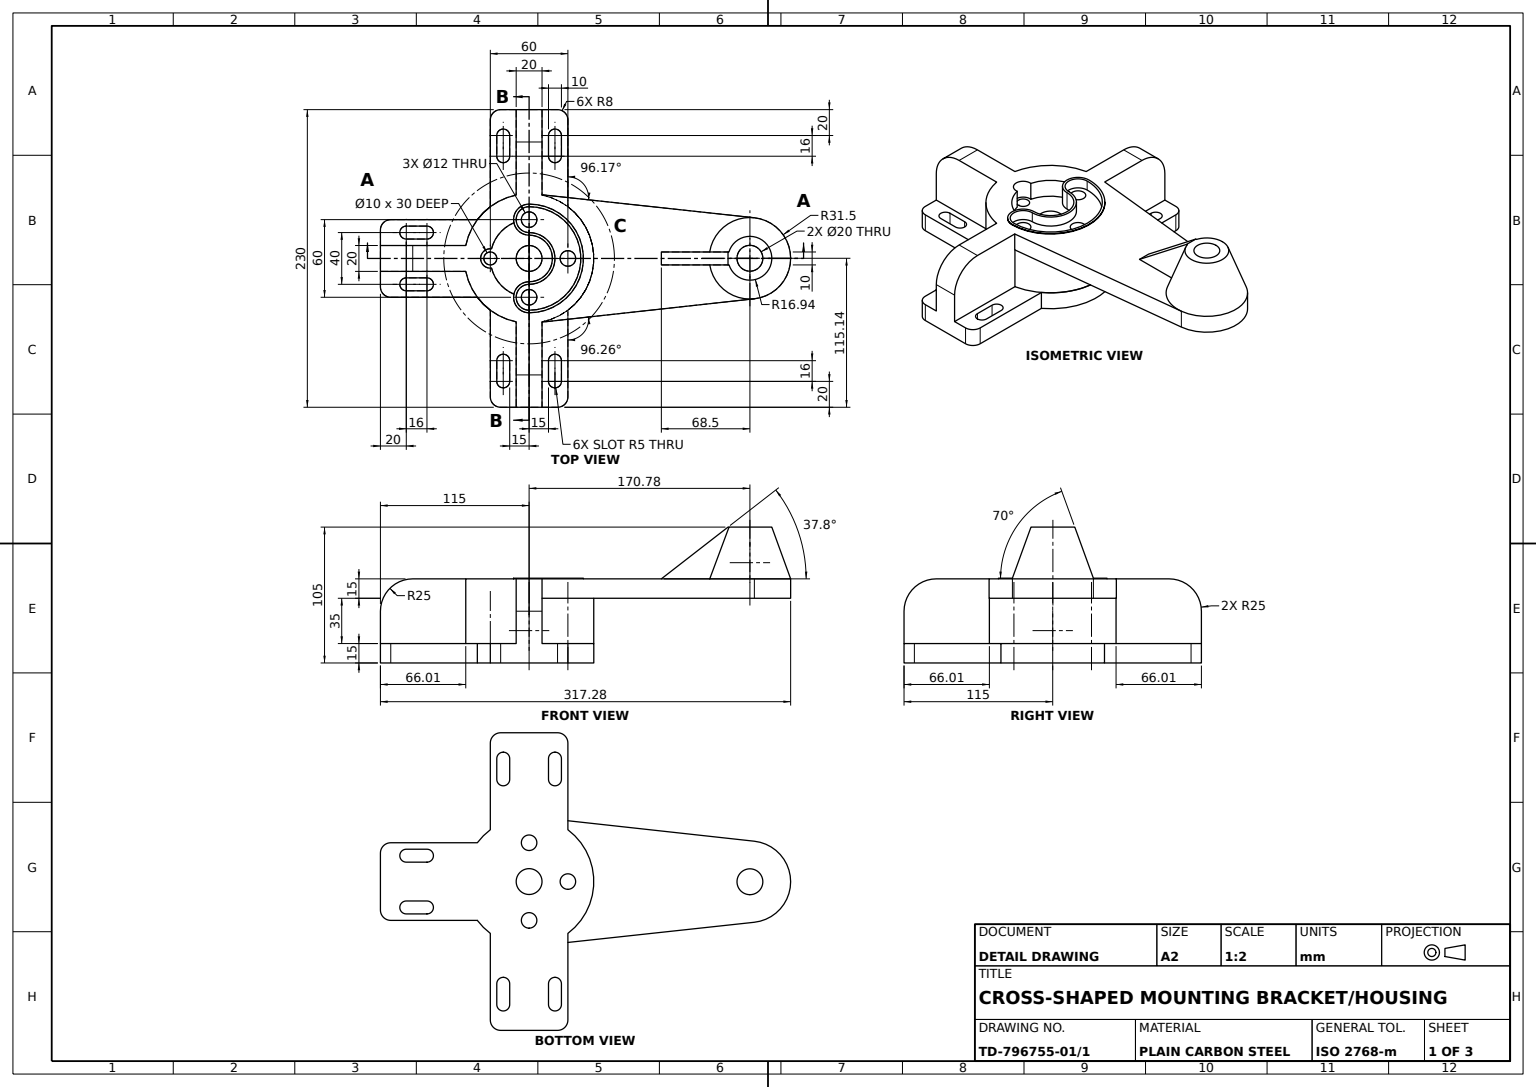
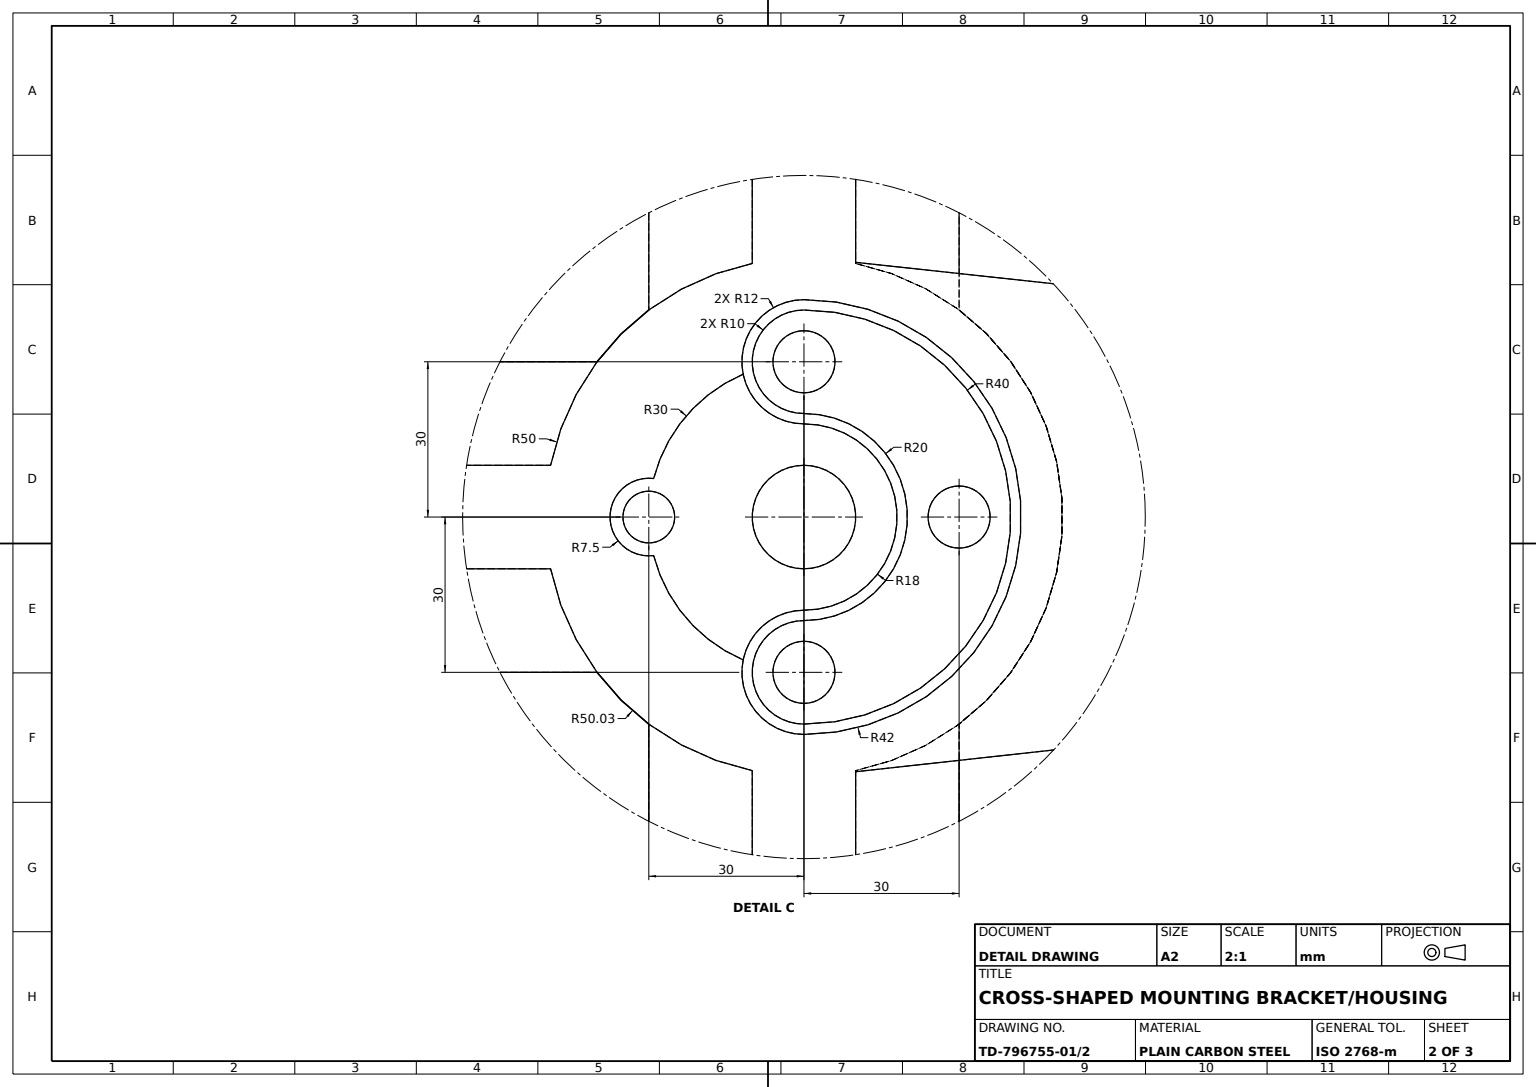
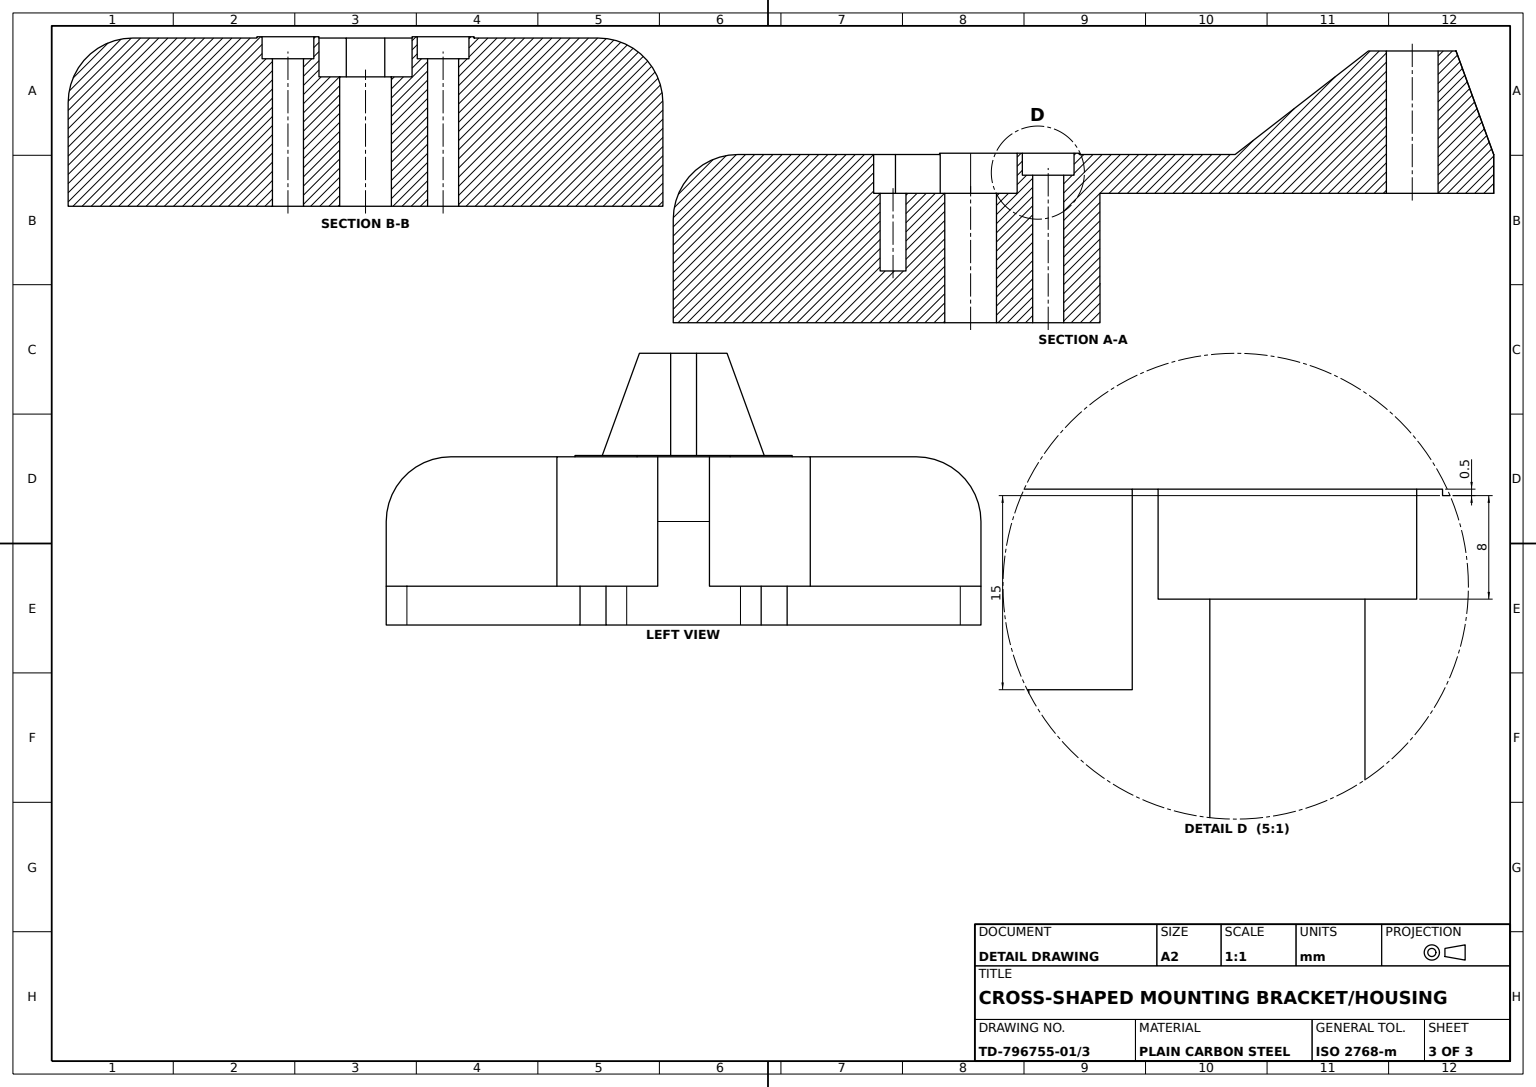
from build123d import *

# Parameters (mm, degrees)
CROSS_BASE_PLATE_SKETCH_R    = 50.034127187
CROSS_BASE_PLATE_DEPTH       = 15
ARM_SLOTS_DEPTH              = 15
CENTRAL_HUB_SKETCH_R         = 50
CENTRAL_HUB_100_DEPTH        = 50
TRUNNION_START               = -15
TRUNNION_ARM_PLATE_DEPTH     = 15
TRUNNION_CONE_SKETCH_R       = 31.5
TRUNNION_CONE_BOSS_DEPTH     = 40
TRUNNION_CONE_BOSS_TAPER     = 20
TRUNNION_BORE_SKETCH_R       = 10
TRUNNION_BORE_20_DEPTH       = 100
TRUNNION_GUSSET_DEPTH        = 5
ARM_UPRIGHT_BLOCK_DEPTH      = 10
ARM_UPRIGHT_BLOCK_PAIR_DEPTH = 10
CENTRAL_BORE_SKETCH_R        = 10
CENTRAL_BORE_20_DEPTH        = 200
HUB_TOP_RECESS_SKETCH_R      = 10
HUB_TOP_RECESS_DEPTH         = 15
HUB_LOBE_POCKET_DEPTH        = 8
POCKET_FLOOR_PAD_DEPTH       = 1
POCKET_START                 = 8.5
POCKET_THIN_WALL_DEPTH       = 8.5
HUB_PIN_HOLES_SKETCH_R       = 6
HUB_PIN_HOLES_DEPTH          = 200
POCKET_OUTER_WALL_DEPTH      = 50
PIN_HOLE_BOSSES_SKETCH_R     = 6
PIN_HOLE_BOSSES_DEPTH        = 20
HUB_SIDE_HOLE_SKETCH_R       = 5
HUB_SIDE_HOLE_10_DEPTH       = 30


with BuildPart() as part:
    # Cross Base Plate Sketch → Cross Base Plate (new body)
    with BuildSketch(Plane(origin=(0, 0, 0), x_dir=(1, 0, 0), z_dir=(0, 1, 0))):
        with BuildLine():
            ThreePointArc((-40.042650803, -30), (-50.034127187, 0), (-40.042650803, 30))
            Line((-40.042650803, 30), (-107, 30))
            ThreePointArc((-107, 30), (-112.656854249, 27.656854249), (-115, 22))
            Line((-115, 22), (-115, -22))
            ThreePointArc((-115, -22), (-112.656854249, -27.656854249), (-107, -30))
            Line((-107, -30), (-40.042650803, -30))
        make_face()
        Circle(CROSS_BASE_PLATE_SKETCH_R)
        with BuildLine():
            ThreePointArc((-30, 40.042650803), (0, 50.034127187), (30, 40.042650803))
            Line((30, 40.042650803), (30, 107))
            ThreePointArc((30, 107), (27.656854249, 112.656854249), (22, 115))
            Line((22, 115), (-22, 115))
            ThreePointArc((-22, 115), (-27.656854249, 112.656854249), (-30, 107))
            Line((-30, 107), (-30, 40.042650803))
        make_face()
        with BuildLine():
            Line((30, -107), (30, -40.042650803))
            ThreePointArc((30, -40.042650803), (0, -50.034127187), (-30, -40.042650803))
            Line((-30, -40.042650803), (-30, -107))
            ThreePointArc((-30, -107), (-27.656854249, -112.656854249), (-22, -115))
            Line((-22, -115), (22, -115))
            ThreePointArc((22, -115), (27.656854249, -112.656854249), (30, -107))
        make_face()
    extrude(amount=CROSS_BASE_PLATE_DEPTH)

    # Arm Slots Sketch → Arm Slots (cut)
    with BuildSketch(Plane(origin=(0, 15, 0), x_dir=(1, 0, 0), z_dir=(0, 1, 0))):
        with BuildLine():
            Line((-95, 25), (-79, 25))
            ThreePointArc((-79, 25), (-74, 20), (-79, 15))
            Line((-79, 15), (-95, 15))
            ThreePointArc((-95, 15), (-100, 20), (-95, 25))
        make_face()
        with BuildLine():
            Line((-95, -25), (-79, -25))
            ThreePointArc((-79, -25), (-74, -20), (-79, -15))
            Line((-79, -15), (-95, -15))
            ThreePointArc((-95, -15), (-100, -20), (-95, -25))
        make_face()
        with BuildLine():
            Line((25, 95), (25, 79))
            ThreePointArc((25, 79), (20, 74), (15, 79))
            Line((15, 79), (15, 95))
            ThreePointArc((15, 95), (20, 100), (25, 95))
        make_face()
        with BuildLine():
            Line((-25, 95), (-25, 79))
            ThreePointArc((-25, 79), (-20, 74), (-15, 79))
            Line((-15, 79), (-15, 95))
            ThreePointArc((-15, 95), (-20, 100), (-25, 95))
        make_face()
        with BuildLine():
            Line((25, -95), (25, -79))
            ThreePointArc((25, -79), (20, -74), (15, -79))
            Line((15, -79), (15, -95))
            ThreePointArc((15, -95), (20, -100), (25, -95))
        make_face()
        with BuildLine():
            Line((-25, -95), (-25, -79))
            ThreePointArc((-25, -79), (-20, -74), (-15, -79))
            Line((-15, -79), (-15, -95))
            ThreePointArc((-15, -95), (-20, -100), (-25, -95))
        make_face()
    extrude(amount=-ARM_SLOTS_DEPTH, mode=Mode.SUBTRACT)

    # Central Hub Sketch → Central Hub Ø100 (add)
    with BuildSketch(Plane(origin=(0, 15, 0), x_dir=(1, 0, 0), z_dir=(0, 1, 0))):
        with Locations(Location((0, 0, 0), (0, 0, 270))):
            Circle(CENTRAL_HUB_SKETCH_R)
    extrude(amount=CENTRAL_HUB_100_DEPTH)

    # Trunnion Arm Plate Sketch → Trunnion Arm Plate (add)
    with BuildSketch(Plane(origin=(0, 65, 0), x_dir=(1, 0, 0), z_dir=(0, 1, 0)).offset(TRUNNION_START)):
        with BuildLine():
            Line((174.172023337, 31.452444757), (5.376852484, 49.710053886))
            ThreePointArc((5.376852484, 49.710053886), (37.207812514, 33.400279758), (50, 0))
            ThreePointArc((50, 0), (37.234224431, -33.370833538), (5.45549876, -49.701484216))
            Line((5.45549876, -49.701484216), (174.221570491, -31.176824248))
            ThreePointArc((174.221570491, -31.176824248), (202.284596415, 0.160031023), (174.172023337, 31.452444757))
        make_face()
    extrude(amount=TRUNNION_ARM_PLATE_DEPTH)

    # Trunnion Cone Sketch → Trunnion Cone Boss (add)
    with BuildSketch(Plane(origin=(0, 65, 0), x_dir=(1, 0, 0), z_dir=(0, 1, 0))):
        with Locations((170.784606272, 0.135110808)):
            Circle(TRUNNION_CONE_SKETCH_R)
    extrude(amount=TRUNNION_CONE_BOSS_DEPTH, taper=TRUNNION_CONE_BOSS_TAPER)

    # Trunnion Bore Sketch → Trunnion Bore Ø20 (cut)
    with BuildSketch(Plane(origin=(0, 105, 0), x_dir=(1, 0, 0), z_dir=(0, 1, 0))):
        with Locations(Location((170.784606272, 0.135110808, 0), (0, 0, 270))):
            Circle(TRUNNION_BORE_SKETCH_R)
    extrude(amount=-TRUNNION_BORE_20_DEPTH, mode=Mode.SUBTRACT)

    # Trunnion Gusset Sketch → Trunnion Gusset (add, symmetric)
    with BuildSketch(Plane.XY):
        Polygon((158.843415643, 65), (102.284606272, 65), (153.843415643, 105), (158.843415643, 105), align=None)
    extrude(amount=TRUNNION_GUSSET_DEPTH, both=True)

    # Arm Upright Block Sketch → Arm Upright Block (add, symmetric)
    with BuildSketch(Plane.XY):
        with BuildLine():
            Line((-115, 15), (-115, 30))
            Line((-115, 30), (-115, 40))
            ThreePointArc((-115, 40), (-107.67766953, 57.67766953), (-90, 65))
            Line((-90, 65), (-42.455555727, 65))
            Line((-42.455555727, 65), (-42.455555727, 15))
            Line((-42.455555727, 15), (-115, 15))
        make_face()
    extrude(amount=ARM_UPRIGHT_BLOCK_DEPTH, both=True)

    # Arm Upright Block Pair Sketch → Arm Upright Block Pair (add, symmetric)
    with BuildSketch(Plane(origin=(0, 0, 0), x_dir=(0, 0, -1), z_dir=(1, 0, 0))):
        with BuildLine():
            Line((115, 15), (115, 40))
            ThreePointArc((115, 40), (107.67766953, 57.67766953), (90, 65))
            Line((90, 65), (40.208016437, 65))
            Line((40.208016437, 65), (40.042650803, 15))
            Line((40.042650803, 15), (115, 15))
        make_face()
        with BuildLine():
            Line((-115, 15), (-115, 40))
            ThreePointArc((-115, 40), (-107.67766953, 57.67766953), (-90, 65))
            Line((-90, 65), (-41.408255734, 65))
            Line((-41.408255734, 65), (-41.408255734, 15))
            Line((-41.408255734, 15), (-115, 15))
        make_face()
    extrude(amount=ARM_UPRIGHT_BLOCK_PAIR_DEPTH, both=True)

    # Central Bore Sketch → Central Bore Ø20 (cut)
    with BuildSketch(Plane(origin=(0, 65, 0), x_dir=(1, 0, 0), z_dir=(0, 1, 0))):
        with Locations(Location((0, 0, 0), (0, 0, 270))):
            Circle(CENTRAL_BORE_SKETCH_R)
    extrude(amount=-CENTRAL_BORE_20_DEPTH, mode=Mode.SUBTRACT)

    # Hub Top Recess Sketch → Hub Top Recess (cut)
    with BuildSketch(Plane(origin=(0, 65, 0), x_dir=(1, 0, 0), z_dir=(0, 1, 0))):
        with BuildLine():
            ThreePointArc((-29.0625, -7.441175562), (30, 0), (-29.0625, 7.441175562))
            ThreePointArc((-29.0625, 7.441175562), (-37.5, 0), (-29.0625, -7.441175562))
        make_face()
        with Locations(Location((0, 0, 0), (0, 0, 270))):
            Circle(HUB_TOP_RECESS_SKETCH_R, mode=Mode.SUBTRACT)
    extrude(amount=-HUB_TOP_RECESS_DEPTH, mode=Mode.SUBTRACT)

    # Hub Lobe Pocket Sketch → Hub Lobe Pocket (cut)
    with BuildSketch(Plane(origin=(0, 65, 0), x_dir=(1, 0, 0), z_dir=(0, 1, 0))):
        with BuildLine():
            ThreePointArc((0, 41), (-11, 30), (0, 19))
            ThreePointArc((0, 19), (19, 0), (0, -19))
            ThreePointArc((0, -19), (-11, -30), (0, -41))
            ThreePointArc((0, -41), (41, 0), (0, 41))
        make_face()
    extrude(amount=-HUB_LOBE_POCKET_DEPTH, mode=Mode.SUBTRACT)

    # Pocket Floor Pad Sketch → Pocket Floor Pad (add)
    with BuildSketch(Plane(origin=(0, 57, 0), x_dir=(1, 0, 0), z_dir=(0, 1, 0))):
        with BuildLine():
            ThreePointArc((0, 41), (-11, 30), (0, 19))
            ThreePointArc((0, 19), (19, 0), (0, -19))
            ThreePointArc((0, -19), (-11, -30), (0, -41))
            ThreePointArc((0, -41), (41, 0), (0, 41))
        make_face()
    extrude(amount=-POCKET_FLOOR_PAD_DEPTH)

    # Pocket Thin Wall Sketch → Pocket Thin Wall (add)
    with BuildSketch(Plane(origin=(0, 57, 0), x_dir=(1, 0, 0), z_dir=(0, 1, 0)).offset(POCKET_START)):
        with BuildLine():
            ThreePointArc((0, 41), (-11, 30), (0, 19))
            ThreePointArc((0, 19), (19, 0), (0, -19))
            ThreePointArc((0, -19), (-11, -30), (0, -41))
            ThreePointArc((0, -41), (41, 0), (0, 41))
        make_face()
        with BuildLine():
            ThreePointArc((0, 40), (-10, 30), (0, 20))
            ThreePointArc((0, 20), (20, 0), (0, -20))
            ThreePointArc((0, -20), (-10, -30), (0, -40))
            ThreePointArc((0, -40), (40, 0), (0, 40))
        make_face(mode=Mode.SUBTRACT)
    extrude(amount=-POCKET_THIN_WALL_DEPTH)

    # Hub Pin Holes Sketch → Hub Pin Holes (cut)
    with BuildSketch(Plane(origin=(0, 57, 0), x_dir=(1, 0, 0), z_dir=(0, 1, 0))):
        with Locations(Location((0, 30, 0), (0, 0, 270))):
            Circle(HUB_PIN_HOLES_SKETCH_R)
        with Locations(Location((30, 0, 0), (0, 0, 270))):
            Circle(HUB_PIN_HOLES_SKETCH_R)
        with Locations(Location((0, -30, 0), (0, 0, 270))):
            Circle(HUB_PIN_HOLES_SKETCH_R)
    extrude(amount=-HUB_PIN_HOLES_DEPTH, mode=Mode.SUBTRACT)

    # Pocket Outer Wall Sketch → Pocket Outer Wall (add)
    with BuildSketch(Plane(origin=(0, 65.5, 0), x_dir=(1, 0, 0), z_dir=(0, 1, 0))):
        with BuildLine():
            ThreePointArc((0, 18), (18, 0), (0, -18))
            ThreePointArc((0, -18), (-12, -30), (0, -42))
            ThreePointArc((0, -42), (42, 0), (0, 42))
            ThreePointArc((0, 42), (-12, 30), (0, 18))
        make_face()
        with BuildLine():
            ThreePointArc((0, 19), (19, 0), (0, -19))
            ThreePointArc((0, -19), (-11, -30), (0, -41))
            ThreePointArc((0, -41), (41, 0), (0, 41))
            ThreePointArc((0, 41), (-11, 30), (0, 19))
        make_face(mode=Mode.SUBTRACT)
    extrude(amount=-POCKET_OUTER_WALL_DEPTH)

    # Pin Hole Bosses Sketch → Pin Hole Bosses (add)
    with BuildSketch(Plane(origin=(0, 57, 0), x_dir=(1, 0, 0), z_dir=(0, 1, 0))):
        with BuildLine():
            ThreePointArc((-10.777754868, -27.8), (-8.520563362, -36.957010852), (0, -41))
            ThreePointArc((0, -41), (41, 0), (0, 41))
            ThreePointArc((0, 41), (-11, 30), (0, 19))
            ThreePointArc((0, 19), (19, 0), (0, -19))
            ThreePointArc((0, -19), (-6.957010852, -21.479436638), (-10.777754868, -27.8))
        make_face()
        with Locations(Location((0, 30, 0), (0, 0, 270))):
            Circle(PIN_HOLE_BOSSES_SKETCH_R, mode=Mode.SUBTRACT)
        with Locations(Location((30, 0, 0), (0, 0, 270))):
            Circle(PIN_HOLE_BOSSES_SKETCH_R, mode=Mode.SUBTRACT)
        with Locations(Location((0, -30, 0), (0, 0, 270))):
            Circle(PIN_HOLE_BOSSES_SKETCH_R, mode=Mode.SUBTRACT)
    extrude(amount=-PIN_HOLE_BOSSES_DEPTH)

    # Hub Side Hole Sketch → Hub Side Hole Ø10 (cut)
    with BuildSketch(Plane(origin=(0, 50, 0), x_dir=(1, 0, 0), z_dir=(0, 1, 0))):
        with Locations(Location((-30, 0, 0), (0, 0, 270))):
            Circle(HUB_SIDE_HOLE_SKETCH_R)
    extrude(amount=-HUB_SIDE_HOLE_10_DEPTH, mode=Mode.SUBTRACT)


solid = part.part
